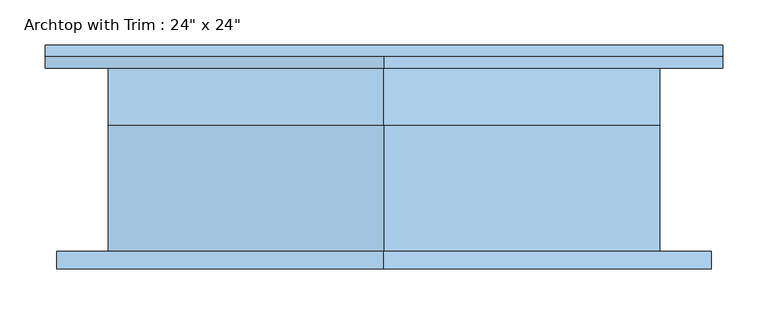
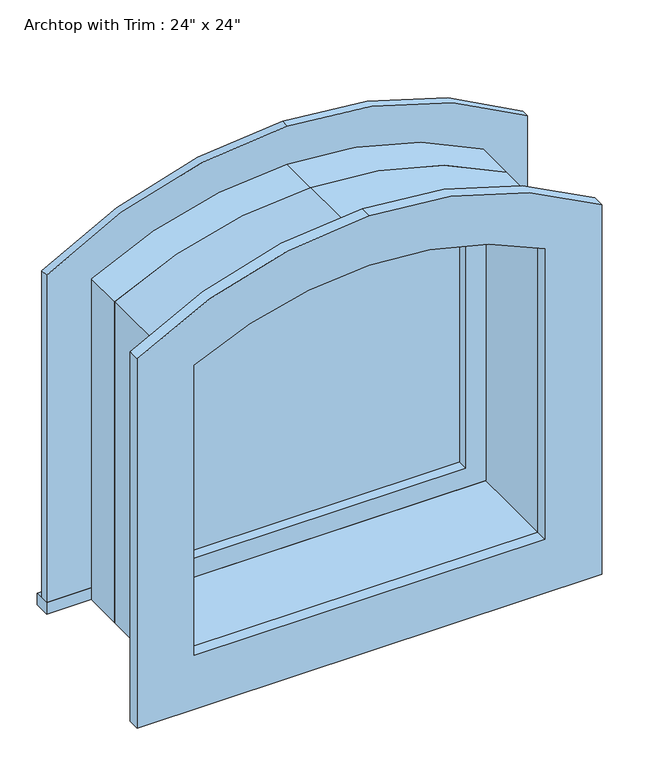
"""IFC4 building model written with IfcOpenShell, lengths in millimetres: window geometry."""

from ifc_helpers import new_model, si_unit, point, frame, frame_2d, origin, place, context, project, spatial, polyline, circle_curve, trimmed, segment, composite_curve, outline, extrude, source, transform, mapped, element, save


def window_08a4fb52(model_context):
    return source(origin(), model_context, "Body", "SweptSolid", [
        extrude(outline(composite_curve([segment(polyline([(946.15, 297.730298), (1431.2135447, 297.730298)]), True, "CONTINUOUS"), segment(trimmed(circle_curve(frame_2d((914.4, 11.980298)), 590.55), [point((1431.2135447, 297.730298))], [point((1504.95, 11.980298))], False, "CARTESIAN"), True, "CONTINUOUS"), segment(trimmed(circle_curve(frame_2d((914.4, 11.980298)), 590.55), [point((1504.95, 11.980298))], [point((1431.2135448, -273.7697019))], False, "CARTESIAN"), True, "CONTINUOUS"), segment(polyline([(1431.2135448, -273.7697019), (946.15, -273.7697019), (946.15, 297.730298)]), True, "CONTINUOUS")], self_intersect=False), holes=[composite_curve([segment(polyline([(977.9, 253.280298), (977.9, -229.319702), (1407.8342262, -229.319702)]), True, "CONTINUOUS"), segment(trimmed(circle_curve(frame_2d((914.4, 11.980298)), 549.275), [point((1407.8342262, -229.319702))], [point((1463.675, 11.980298))], True, "CARTESIAN"), True, "CONTINUOUS"), segment(trimmed(circle_curve(frame_2d((914.4, 11.980298)), 549.275), [point((1463.675, 11.980298))], [point((1407.8342262, 253.280298))], True, "CARTESIAN"), True, "CONTINUOUS"), segment(polyline([(1407.8342262, 253.280298), (977.9, 253.280298)]), True, "CONTINUOUS")], self_intersect=False)]), frame((0.0, 38.1, 0.0), z_axis=(0.0, 1.0, 0.0), x_axis=(0.0, 0.0, 1.0)), (0.0, 0.0, 1.0), 44.45),
        extrude(outline(polyline([(-362.6697019, 127.0), (386.630298, 127.0), (386.630298, 101.6), (-362.6697019, 101.6), (-362.6697019, 127.0)])), frame((0.0, 0.0, 914.4), z_axis=(0.0, 0.0, 1.0), x_axis=(1.0, 0.0, 0.0)), (0.0, 0.0, 1.0), 19.05),
        extrude(outline(composite_curve([segment(polyline([(933.45, 297.7302979), (933.45, 386.630298), (1472.3420964, 386.630298)]), True, "CONTINUOUS"), segment(trimmed(circle_curve(frame_2d((914.4, 11.980298)), 672.0580373), [point((1472.3420964, 386.630298))], [point((1586.4580373, 11.980298))], False, "CARTESIAN"), True, "CONTINUOUS"), segment(trimmed(circle_curve(frame_2d((914.4, 11.980298)), 672.0580373), [point((1586.4580373, 11.980298))], [point((1472.3420965, -362.6697019))], False, "CARTESIAN"), True, "CONTINUOUS"), segment(polyline([(1472.3420965, -362.6697019), (933.45, -362.6697019), (933.45, -273.7697019), (1431.2135447, -273.7697019)]), True, "CONTINUOUS"), segment(trimmed(circle_curve(frame_2d((914.4, 11.980298)), 590.55), [point((1431.2135447, -273.7697019))], [point((1504.95, 11.980298))], True, "CARTESIAN"), True, "CONTINUOUS"), segment(trimmed(circle_curve(frame_2d((914.4, 11.980298)), 590.55), [point((1504.95, 11.980298))], [point((1431.2135448, 297.7302979))], True, "CARTESIAN"), True, "CONTINUOUS"), segment(polyline([(1431.2135448, 297.7302979), (933.45, 297.7302979)]), True, "CONTINUOUS")], self_intersect=False)), frame((0.0, 101.6, 0.0), z_axis=(0.0, 1.0, 0.0), x_axis=(0.0, 0.0, 1.0)), (0.0, 0.0, 1.0), 12.7),
        extrude(outline(composite_curve([segment(polyline([(857.25, -349.969702), (857.25, 373.9302979), (1465.1014713, 373.9302979)]), True, "CONTINUOUS"), segment(trimmed(circle_curve(frame_2d((914.4, 11.980298)), 658.9991752), [point((1465.1014713, 373.9302979))], [point((1573.3991752, 11.980298))], False, "CARTESIAN"), True, "CONTINUOUS"), segment(trimmed(circle_curve(frame_2d((914.4, 11.980298)), 658.9991752), [point((1573.3991752, 11.980298))], [point((1465.1014713, -349.969702))], False, "CARTESIAN"), True, "CONTINUOUS"), segment(polyline([(1465.1014713, -349.969702), (857.25, -349.969702)]), True, "CONTINUOUS")], self_intersect=False), holes=[composite_curve([segment(polyline([(946.15, -261.0697027), (1423.6684161, -261.0697027)]), True, "CONTINUOUS"), segment(trimmed(circle_curve(frame_2d((914.4, 11.980298)), 577.85), [point((1423.6684161, -261.0697027))], [point((1492.25, 11.980298))], True, "CARTESIAN"), True, "CONTINUOUS"), segment(trimmed(circle_curve(frame_2d((914.4000002, 11.980298)), 577.8499998), [point((1492.25, 11.980298))], [point((1423.6684161, 285.0302987))], True, "CARTESIAN"), True, "CONTINUOUS"), segment(polyline([(1423.6684161, 285.0302987), (946.15, 285.0302987), (946.15, -261.0697027)]), True, "CONTINUOUS")], self_intersect=False)]), frame((0.0, -120.65, 0.0), z_axis=(0.0, 1.0, 0.0), x_axis=(0.0, 0.0, 1.0)), (0.0, 0.0, 1.0), 19.05),
        extrude(outline(composite_curve([segment(polyline([(977.9, -229.3197017), (977.9, 253.2802981), (1408.1281367, 253.2802981)]), True, "CONTINUOUS"), segment(trimmed(circle_curve(frame_2d((914.4, 11.9802983)), 549.5390458), [point((1408.1281367, 253.2802981))], [point((1463.9390458, 11.9802983))], False, "CARTESIAN"), True, "CONTINUOUS"), segment(trimmed(circle_curve(frame_2d((914.4, 11.9802983)), 549.5390458), [point((1463.9390458, 11.9802983))], [point((1408.1281366, -229.3197017))], False, "CARTESIAN"), True, "CONTINUOUS"), segment(polyline([(1408.1281366, -229.3197017), (977.9, -229.3197017)]), True, "CONTINUOUS")], self_intersect=False)), frame((0.0, 53.975, 0.0), z_axis=(0.0, 1.0, 0.0), x_axis=(0.0, 0.0, 1.0)), (0.0, 0.0, 1.0), 12.7),
        extrude(outline(composite_curve([segment(polyline([(914.4, 316.780298), (1442.3290861, 316.780298)]), True, "CONTINUOUS"), segment(trimmed(circle_curve(frame_2d((914.4, 11.980298)), 609.6), [point((1442.3290861, 316.780298))], [point((1524.0, 11.980298))], False, "CARTESIAN"), True, "CONTINUOUS"), segment(trimmed(circle_curve(frame_2d((914.4, 11.980298)), 609.6), [point((1524.0, 11.980298))], [point((1442.3290861, -292.819702))], False, "CARTESIAN"), True, "CONTINUOUS"), segment(polyline([(1442.3290861, -292.819702), (914.4, -292.819702), (914.4, 316.780298)]), True, "CONTINUOUS")], self_intersect=False), holes=[composite_curve([segment(polyline([(946.15, 285.0302987), (946.15, -261.069702), (1427.2825062, -261.069702)]), True, "CONTINUOUS"), segment(trimmed(circle_curve(frame_2d((914.4, 11.980298)), 581.0376646), [point((1427.2825062, -261.069702))], [point((1495.4376646, 11.980298))], True, "CARTESIAN"), True, "CONTINUOUS"), segment(trimmed(circle_curve(frame_2d((914.4, 11.980298)), 581.0376646), [point((1495.4376646, 11.980298))], [point((1427.2825058, 285.0302987))], True, "CARTESIAN"), True, "CONTINUOUS"), segment(polyline([(1427.2825058, 285.0302987), (946.15, 285.0302987)]), True, "CONTINUOUS")], self_intersect=False)]), frame((0.0, -101.6, 0.0), z_axis=(0.0, 1.0, 0.0), x_axis=(0.0, 0.0, 1.0)), (0.0, 0.0, 1.0), 139.7),
        extrude(outline(composite_curve([segment(polyline([(914.4, -292.819702), (914.4, 316.780298), (1442.3290861, 316.780298)]), True, "CONTINUOUS"), segment(trimmed(circle_curve(frame_2d((914.4, 11.980298)), 609.6), [point((1442.3290861, 316.780298))], [point((1524.0, 11.980298))], False, "CARTESIAN"), True, "CONTINUOUS"), segment(trimmed(circle_curve(frame_2d((914.4, 11.980298)), 609.6), [point((1524.0, 11.980298))], [point((1442.3290861, -292.819702))], False, "CARTESIAN"), True, "CONTINUOUS"), segment(polyline([(1442.3290861, -292.819702), (914.4, -292.819702)]), True, "CONTINUOUS")], self_intersect=False), holes=[composite_curve([segment(polyline([(933.45, -273.7697019), (1433.3358634, -273.7697019)]), True, "CONTINUOUS"), segment(trimmed(circle_curve(frame_2d((914.4, 11.980298)), 592.4082147), [point((1433.3358634, -273.7697019))], [point((1506.8082147, 11.980298))], True, "CARTESIAN"), True, "CONTINUOUS"), segment(trimmed(circle_curve(frame_2d((914.4, 11.980298)), 592.4082147), [point((1506.8082147, 11.980298))], [point((1433.3358634, 297.730298))], True, "CARTESIAN"), True, "CONTINUOUS"), segment(polyline([(1433.3358634, 297.730298), (933.45, 297.730298), (933.45, -273.7697019)]), True, "CONTINUOUS")], self_intersect=False)]), frame((0.0, 38.1, 0.0), z_axis=(0.0, 1.0, 0.0), x_axis=(0.0, 0.0, 1.0)), (0.0, 0.0, 1.0), 63.5),
    ])


if __name__ == "__main__":
    model = new_model("IFC4")
    model_context = context("Model", 3, world=origin())
    ifc_project = project(units=[si_unit("LENGTHUNIT", "METRE", prefix="MILLI")], contexts=[model_context])
    site = spatial("IfcSite", under=ifc_project)
    building = spatial("IfcBuilding", under=site)
    placement = place(None, origin())
    window_shape = window_08a4fb52(model_context)
    element("IfcWindow", 1, ObjectType="Archtop with Trim : 24\" x 24\"", at=placement, inside=building, context=model_context, shape_type="MappedRepresentation", body=[
        mapped(window_shape, transform((0.0, 0.0, 0.0), x_axis=(1.0, 0.0, 0.0), y_axis=(0.0, 1.0, 0.0), z_axis=(0.0, 0.0, 1.0))),
    ])
    save(model, "model.ifc")

# Revit data of these elements
# Type "Archtop with Trim : 24\" x 24\""
#   Type Mark = "15"
#   Construction Type Id = "GSP4R"
#   Assembly Code = "B2020100"
#   Analytic Construction = "1/8 in Pilkington single glazing"
#   Visual Light Transmittance = 0.9
#   Solar Heat Gain Coefficient = 0.78
#   Heat Transfer Coefficient (U) = 0.6496 BTU/(h·ft²·°F)
#   Height = 2' - 0"
#   Radius = 2' - 0"
#   Default Sill Height = 3' - 0"
#   Trim Projection - Ext. = 0' - 0 1/2"
#   Trim Projection - Int. = 0' - 0 3/4"
#   Trim Width - Exterior = 0' - 3 1/2"
#   Trim Width - Interior = 0' - 3 1/2"
#   Width = 2' - 0"
#   Define Thermal Properties by = 1
#   Glass Pane Material = Glass
#   Sash Material = Sash
#   Trim Exterior Material = Trim
#   Trim Interior Material = Trim
#   Wall Closure = (empty or 0)
# Element 1 (IfcWindow, "Archtop with Trim : 24\" x 24\"")
#   Materials on its faces: "Sash", "Trim", "Glass"
# Materials
#   "Glass": class "Glass", colour RGB 0 128 192, transparency 0.75, Description = "Soda Lime Glass", Cost = 0
#   "Sash": class "Wood", colour RGB 224 178 126, transparency 0
#   "Trim": class "Wood", colour RGB 224 178 126, transparency 0
